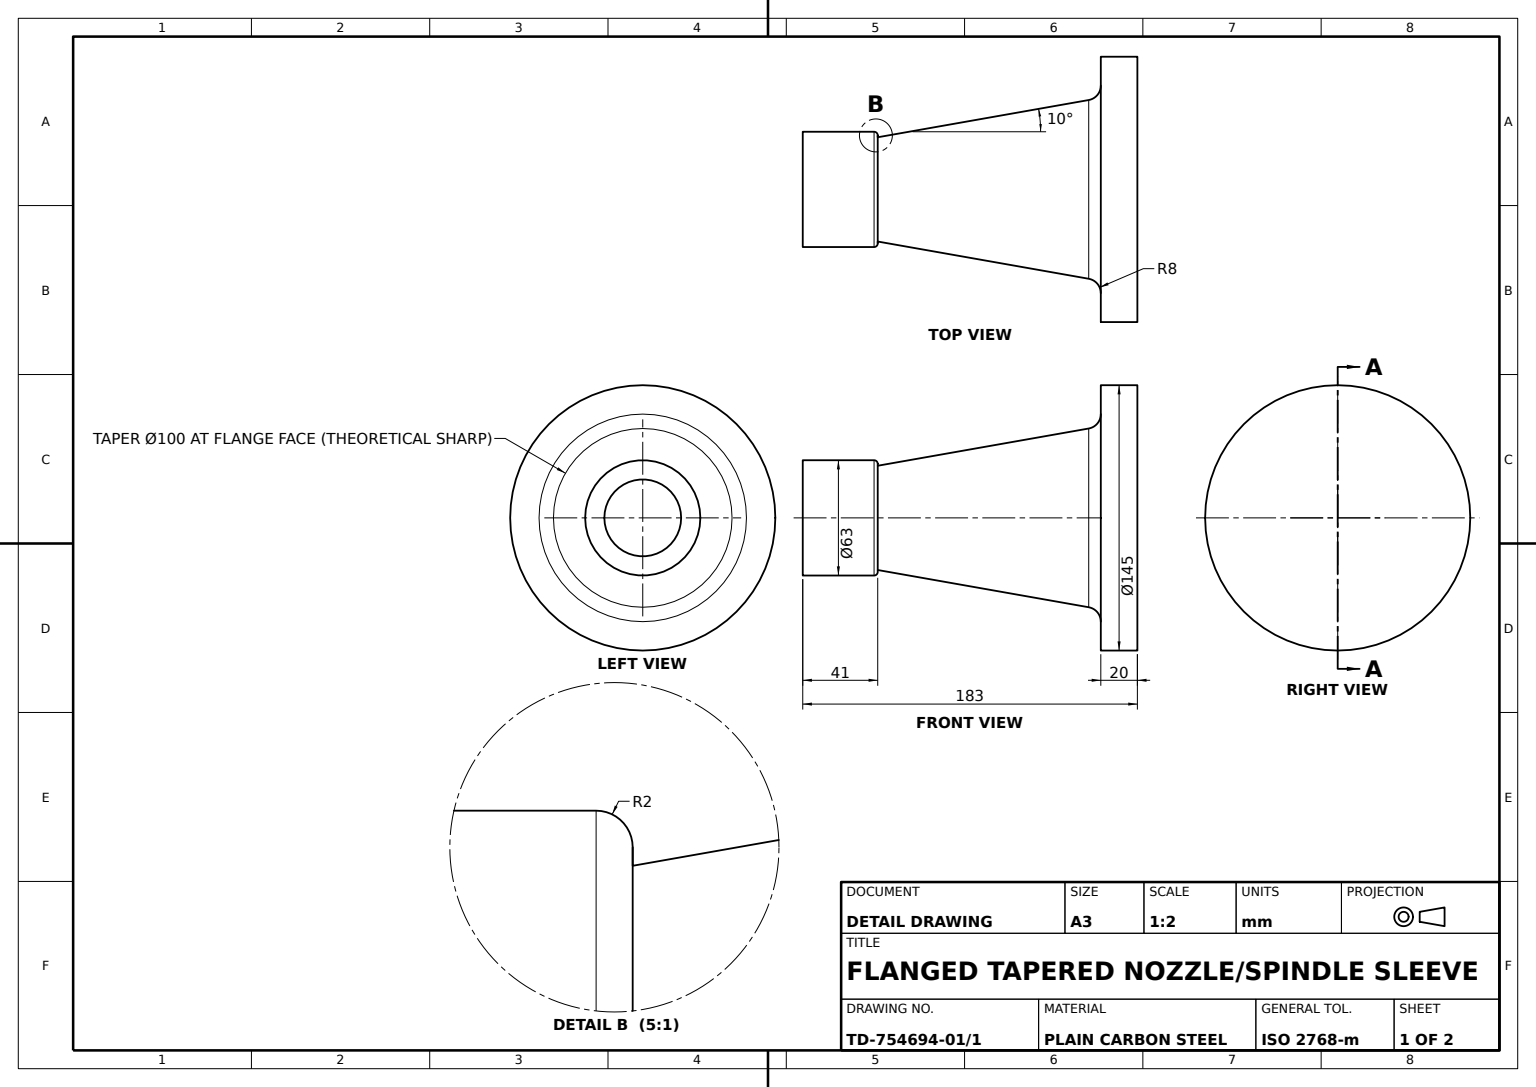
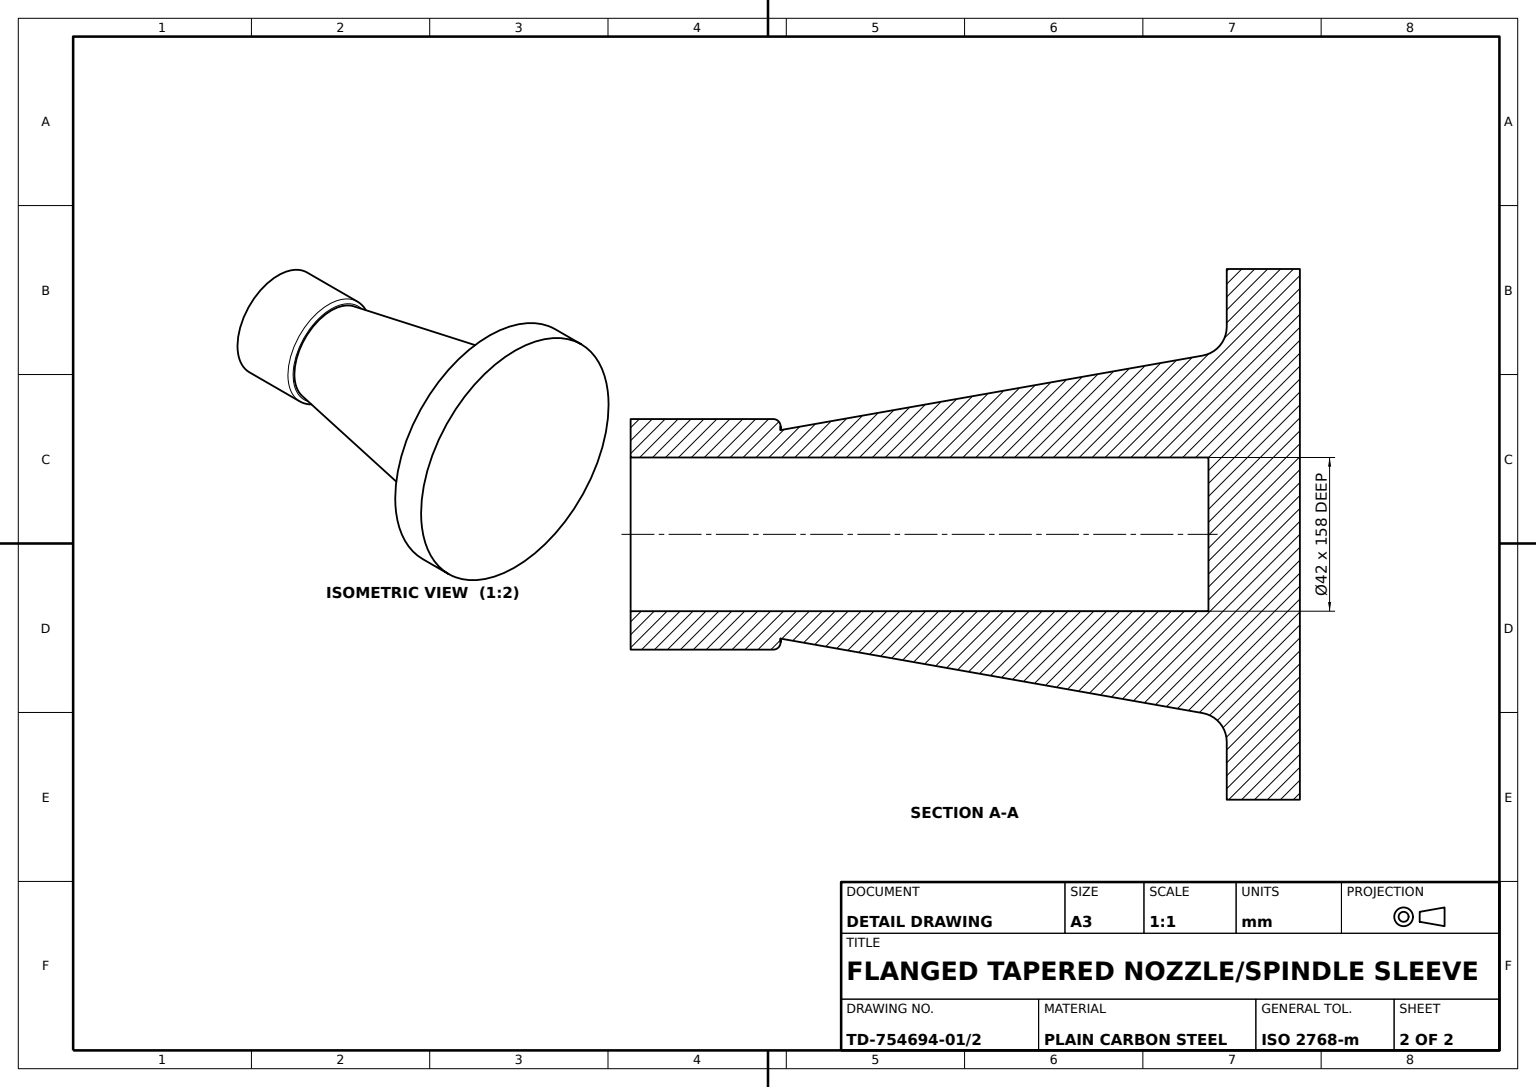
SolidWorks part; units mm, degrees
material "Plain Carbon Steel"
ref_plane "Front Plane" through (0, 0, 0) normal (0, 0, 1) x (1, 0, 0)
ref_plane "Top Plane" through (0, 0, 0) normal (0, 1, 0) x (1, 0, 0)
ref_plane "Right Plane" through (0, 0, 0) normal (1, 0, 0) x (0, 0, -1)
sketch "Flange Sketch Ø145" plane through (0, 0, 0) normal (0, 0, 1) x (1, 0, 0)
  circle A0 centre (0, 0) radius 72.5
  dimension "D1" = 145
extrude "Flange Ø145x20" add sketch "Flange Sketch Ø145" along normal blind 20
sketch "Taper Sketch Ø100" plane through (0, 0, 20) normal (0, 0, 1) x (1, 0, 0)
  circle A0 centre (0, 0) radius 50
  dimension "D1" = 100
extrude "Tapered Body Ø100 10deg Draft" add sketch "Taper Sketch Ø100" along normal blind 125 draft 10
sketch "Spigot Sketch Ø63" plane through (0, 0, 145) normal (0, 0, 1) x (1, 0, 0)
  circle A0 centre (0, 0) radius 31.5
  dimension "D1" = 63
extrude "Spigot Ø63x38" add sketch "Spigot Sketch Ø63" along normal blind 38 and the other way blind 3
sketch "Bore Sketch Ø42" plane through (0, 0, 183) normal (0, 0, 1) x (1, 0, 0)
  circle A0 centre (0, 0) radius 21
  dimension "D1" = 42
extrude "Bore Ø42x158" cut sketch "Bore Sketch Ø42" against normal blind 158
fillet "Flange Root Fillet R8" radius 8 1 edges at (50, 0, 20)
fillet "Spigot Edge Fillet R2" radius 2 1 edges at (31.5, 0, 142)
